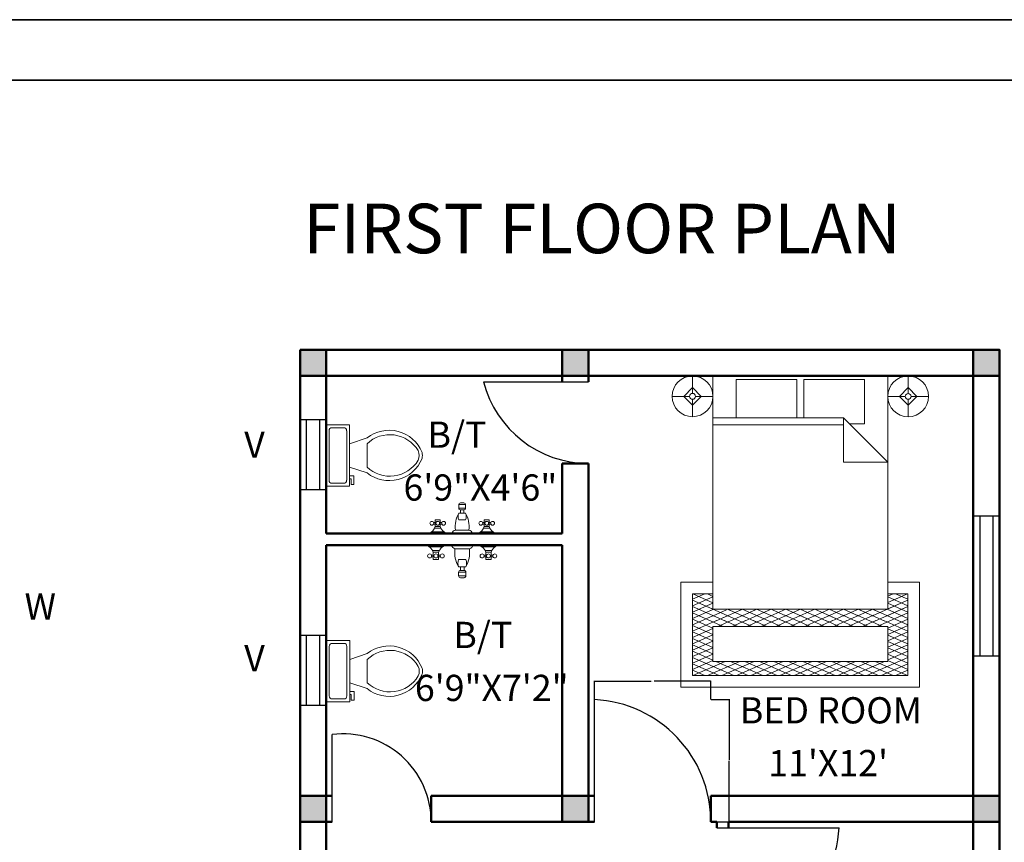
# Model space of a CAD drawing. Units: inches. Extents: x 28637 to 29820, y 17246 to 17928.
# Tile 5 of 6: x 28996 to 29334, y 17646 to 17928. Entities that reach past the tile are written whole.
import ezdxf

# ---------------------------------------------------------------- set-up
doc = ezdxf.new("R2010")
doc.units = ezdxf.units.IN
for name, color, linetype, lineweight in [('A-ANNO-DIMS', 2, 'Continuous', 18), ('A-ANNO-TEXT', 7, 'Continuous', 25), ('A-ANNO-TTLB', 7, 'Continuous', 35), ('A-AREA-IDEN', 30, 'Continuous', 25), ('A-COLS', 1, 'Continuous', 50), ('A-DOOR', 4, 'Continuous', 25), ('A-FLOR-FIXT', 8, 'Continuous', 18), ('A-FURN', 8, 'Continuous', 18), ('A-GLAZ', 4, 'Continuous', 25), ('A-WALL', 7, 'Continuous', 50)]:
    doc.layers.add(name, color=color, linetype=linetype, lineweight=lineweight)
doc.styles.get("Standard").update_dxf_attribs({"font": 'arial.ttf'})
doc.dimstyles.get("Standard").update_dxf_attribs({"dimtxt": 0.18, "dimasz": 0.18, "dimexe": 0.18, "dimexo": 0.0625, "dimgap": 0.09, "dimtad": 0, "dimtih": 1, "dimtoh": 1, "dimdec": 4, "dimzin": 0, "dimdsep": 46, "dimtxsty": 'Standard', "dimcen": 0.09, "dimadec": 0, "dimazin": 0, "dimtfac": 1, "dimtdec": 4, "dimtofl": 0, "dimtmove": 0, "dimatfit": 3, "dimfxl": 1, "dimtolj": 1, "dimtzin": 0, "dimarcsym": 0})

# ---------------------------------------------------------------- blocks, each defined once
blk = doc.blocks.new('Bed - Queen')
for p, q in [((0, -80.00003), (0, 0)), ((0, 0), (59.99999, 0)), ((59.99999, 0), (59.99999, -80.00003)), ((7.99999, -1.2), (28.79998, -1.2)), ((7.99999, -14.4), (7.99999, -1.2)), ((28.79998, -1.2), (28.79998, -14.4)), ((31.19999, -1.2), (51.99999, -1.2)), ((31.19999, -14.4), (31.19999, -1.2)), ((51.99999, -1.2), (51.99999, -16.4)), ((0, -14.4), (44.8, -14.4)), ((44.8, -16.8), (0, -16.8)), ((59.99999, -29.6), (44.8, -14.4)), ((44.8, -14.4), (44.8, -29.6)), ((51.99999, -16.4), (46.79936, -16.4)), ((44.8, -29.6), (59.99999, -29.6)), ((59.99999, -80.00003), (0, -80.00003))]:
    blk.add_line(p, q)
blk = doc.blocks.new('Lamp - Table')
for p, q in [((0, 7), (0, 1)), ((-1, 0), (-7, 0)), ((0, 3), (-3, 0)), ((-3, 0), (0, -3)), ((3, 0), (0, 3)), ((0, -3), (3, 0)), ((1, 0), (7, 0)), ((0, -1), (0, -7))]:
    blk.add_line(p, q)
for radius in [7, 1]:
    blk.add_circle((0, 0), radius)
blk = doc.blocks.new('Toilet - top')
for p, q in [((9.5, -6), (9.5, -2)), ((-10, -8.5), (-8, -8.5)), ((-10, -9.5), (-10, -8.5)), ((-7, -9.5), (-10, -9.5)), ((-8, -8.5), (-8, -8)), ((-7, -8), (-7, -9.5)), ((-4, -8), (-6, -14)), ((4, -8), (6, -14)), ((4, -14), (-4, -14))]:
    blk.add_line(p, q)
blk.add_lwpolyline([(10.5, -8), (10.5, 0), (-10.5, 0), (-10.5, -8)], close=True)
for points in [[(-9.5, -2), (-9.5, -6)], [(8.5, -1), (-8.5, -1)], [(-8.5, -7), (8.5, -7)]]:
    blk.add_lwpolyline(points)
for centre, radius, start, end in [((-8.62, -1.88), 0.884, 81.8699, 188.1301), ((8.62, -1.88), 0.884, 351.8699, 98.1301), ((-8.62, -6.12), 0.884, 171.8699, 278.1301), ((8.62, -6.12), 0.884, 261.8699, 8.1301), ((3.52, -21.58), 12.17, 141.4691, 247.9714), ((4.2, -21.82), 11.33, 136.3677, 238.9468), ((-3.52, -21.58), 12.17, 292.0284, 38.5307), ((-4.2, -21.82), 11.33, 301.053, 43.6321), ((0, -27.88), 4, 245.7318, 294.2682), ((0, -29), 4, 254.8605, 285.1395)]:
    blk.add_arc(centre, radius, start, end)
blk = doc.blocks.new('Faucet - Bathroom front')
for p, q in [((-0.5, 4.25), (0.5, 4.25)), ((0.5, 3.75), (-0.5, 3.75)), ((-0.5, 3), (0.5, 3)), ((-0.25, 3), (-0.25, 3.5)), ((0.25, 3.5), (0.25, 3)), ((-4, 1.625), (-4.25, 1.625)), ((-4, 1.375), (-4.25, 1.375)), ((-3.25, 1.625), (-3, 1.625)), ((-3.25, 1.375), (-3, 1.375)), ((0.5, 2), (-0.5, 2)), ((3.25, 1.625), (3, 1.625)), ((3.25, 1.375), (3, 1.375)), ((4, 1.625), (4.25, 1.625)), ((4, 1.375), (4.25, 1.375)), ((-5, 0), (-2.25, 0)), ((-4.5087, 0.25), (-2.7408, 0.25)), ((-3.1442, 0.75), (-4.0979, 0.75)), ((-1.5, 0), (1.5, 0)), ((-1, 0.5), (1, 0.5)), ((2.25, 0), (5, 0)), ((2.7413, 0.25), (4.5092, 0.25)), ((4.1058, 0.75), (3.1521, 0.75))]:
    blk.add_line(p, q)
for points in [[(-0.5, 3.75), (-0.5, 4.25)], [(-0.25, 4.5), (0.25, 4.5)], [(0.5, 4.25), (0.5, 3.75)], [(0.25, 3.5), (-0.25, 3.5)]]:
    blk.add_lwpolyline(points)
for points in [[(-4, 1), (-4, 2), (-3.25, 2), (-3.25, 1)], [(3.25, 1), (3.25, 2), (4, 2), (4, 1)]]:
    blk.add_lwpolyline(points, close=True)
for centre in [(-4.5, 1.5), (-3.625, 1.5), (-2.75, 1.5), (2.75, 1.5), (3.625, 1.5), (4.5, 1.5)]:
    blk.add_circle(centre, 0.2795)
for centre, radius, start, end in [((-0.2575, 4.2575), 0.2426, 88.22243, 181.7776), ((0.2575, 4.2575), 0.2426, 358.2224, 91.77757), ((3, 1), 4.0311, 150.2551, 187.125), ((0.6413, 2.5), 1.246, 156.3417, 203.6583), ((-0.2575, 3.7425), 0.2426, 178.2224, 271.7776), ((0.2575, 3.7425), 0.2426, 268.2224, 1.777565), ((-3, 1), 4.0311, 352.875, 29.74488), ((-0.6413, 2.5), 1.246, 336.3417, 23.65835), ((-5.375, 1.375), 1.4252, 285.2551, 344.7449), ((-1.875, 1.375), 1.4252, 195.2551, 254.7449), ((-0.7962, -0.2038), 0.7327, 106.1502, 163.8498), ((0.7962, -0.2038), 0.7327, 16.1502, 73.84979), ((1.875, 1.375), 1.4252, 285.2551, 344.7449), ((5.375, 1.375), 1.4252, 195.2551, 254.7449)]:
    blk.add_arc(centre, radius, start, end)
blk = doc.blocks.new('DOOR-42')
blk.add_line((28900.64, 17650.75), (28942.64, 17650.75))
blk.add_arc((28900.64, 17652.8), 42.05, 270, 357.2056)
blk = doc.blocks.new('DOOR-37')
blk.add_line((28816.64, 17803.75), (28852.64, 17803.75))
blk.add_arc((28852.64, 17812.9), 37.14, 194.25, 270)
blk = doc.blocks.new('DOOR-30')
blk.add_line((28764.64, 17652.75), (28764.64, 17682.75))
blk.add_arc((28768.41, 17652.75), 30.24, 0, 97.1527)
blk = doc.blocks.new('*D36')
at = {"layer": 'A-ANNO-DIMS', "color": 0, "lineweight": -2, "transparency": 16777216}
for p, q in [((29232.93, 17694.75), (29239.35, 17694.75)), ((29239.17, 17694.57), (29239.17, 17673.94)), ((29239.17, 17652.93), (29239.17, 17673.57)), ((29232.93, 17652.75), (29239.35, 17652.75))]:
    blk.add_line(p, q, dxfattribs=at)
at = {"layer": 'A-ANNO-DIMS', "color": 0, "transparency": 16777216}
for points in [[(29239.14, 17694.57), (29239.2, 17694.57), (29239.17, 17694.75)], [(29239.14, 17652.93), (29239.2, 17652.93), (29239.17, 17652.75)]]:
    blk.add_solid(points, dxfattribs=at)
at = {"layer": 'Defpoints', "color": 0, "transparency": 16777216}
for p in [(29232.87, 17694.75), (29239.17, 17694.75), (29232.87, 17652.75)]:
    blk.add_point(p, dxfattribs=at)
at = {"layer": 'A-ANNO-DIMS', "color": 0, "transparency": 16777216, "insert": (29239.17, 17673.75), "char_height": 0.18, "attachment_point": 5}
blk.add_mtext('\\A1;DOOR 42 TYP.', dxfattribs=at)
blk = doc.blocks.new('*D37')
at = {"layer": 'A-ANNO-DIMS', "color": 0, "lineweight": -2, "transparency": 16777216}
for p, q in [((29192.87, 17694.81), (29192.87, 17701.23)), ((29193.05, 17701.05), (29212.34, 17701.05)), ((29232.69, 17701.05), (29213.4, 17701.05)), ((29232.87, 17694.81), (29232.87, 17701.23))]:
    blk.add_line(p, q, dxfattribs=at)
at = {"layer": 'A-ANNO-DIMS', "color": 0, "transparency": 16777216}
for points in [[(29193.05, 17701.08), (29193.05, 17701.02), (29192.87, 17701.05)], [(29232.69, 17701.08), (29232.69, 17701.02), (29232.87, 17701.05)]]:
    blk.add_solid(points, dxfattribs=at)
at = {"layer": 'Defpoints', "color": 0, "transparency": 16777216}
for p in [(29192.87, 17701.05), (29192.87, 17694.75), (29232.87, 17694.75)]:
    blk.add_point(p, dxfattribs=at)
at = {"layer": 'A-ANNO-DIMS', "color": 0, "transparency": 16777216, "insert": (29212.87, 17701.05), "char_height": 0.18, "attachment_point": 5}
blk.add_mtext('\\A1;40 TYP.', dxfattribs=at)

msp = doc.modelspace()

# ---------------------------------------------------------------- hatches: boundary and pattern name
at = {"layer": 'A-COLS'}
h = msp.add_hatch(color=256, dxfattribs=at)
h.dxf.hatch_style = 1
h.paths.add_polyline_path([(29091.87, 17814.75), (29091.87, 17805.75), (29100.87, 17805.75), (29100.87, 17814.75)])
h = msp.add_hatch(color=256, dxfattribs=at)
h.dxf.hatch_style = 1
h.paths.add_polyline_path([(29181.87, 17814.75), (29181.87, 17805.75), (29190.87, 17805.75), (29190.87, 17814.75)])
h = msp.add_hatch(color=256, dxfattribs=at)
h.dxf.hatch_style = 1
h.paths.add_polyline_path([(29331.87, 17814.75), (29322.87, 17814.75), (29322.87, 17805.75), (29331.87, 17805.75)])
h = msp.add_hatch(color=256, dxfattribs=at)
h.dxf.hatch_style = 1
h.paths.add_polyline_path([(29091.87, 17661.75), (29091.87, 17652.75), (29100.87, 17652.75), (29100.87, 17661.75)])
h = msp.add_hatch(color=256, dxfattribs=at)
h.dxf.hatch_style = 1
h.paths.add_polyline_path([(29181.87, 17661.75), (29181.87, 17652.75), (29190.87, 17652.75), (29190.87, 17661.75)])
h = msp.add_hatch(color=256, dxfattribs=at)
h.dxf.hatch_style = 1
h.paths.add_polyline_path([(29322.87, 17661.75), (29322.87, 17652.75), (29331.87, 17652.75), (29331.87, 17661.75)])

# ---------------------------------------------------------------- linework, layer by layer
at = {"layer": 'A-ANNO-TTLB'}
for points in [[(28637.03, 17927.97), (29820.02, 17927.97), (29820.02, 17246.37), (28637.03, 17246.37)], [(28663.78, 17907.18), (29794.75, 17907.18), (29794.75, 17268.65), (28663.78, 17268.65)]]:
    msp.add_lwpolyline(points, close=True, dxfattribs=at)
at = {"layer": 'A-COLS'}
for points in [[(29091.87, 17814.75), (29100.87, 17814.75), (29100.87, 17805.75), (29091.87, 17805.75)], [(29181.87, 17814.75), (29190.87, 17814.75), (29190.87, 17805.75), (29181.87, 17805.75)], [(29322.87, 17814.75), (29331.87, 17814.75), (29331.87, 17805.75), (29322.87, 17805.75)], [(29091.87, 17661.75), (29100.87, 17661.75), (29100.87, 17652.75), (29091.87, 17652.75)], [(29181.87, 17661.75), (29190.87, 17661.75), (29190.87, 17652.75), (29181.87, 17652.75)], [(29322.87, 17661.75), (29331.87, 17661.75), (29331.87, 17652.75), (29322.87, 17652.75)]]:
    msp.add_lwpolyline(points, close=True, dxfattribs=at)
at = {"layer": 'A-FURN'}
for p, q in [((29222.57, 17734.98), (29233.57, 17734.98)), ((29222.57, 17734.98), (29222.57, 17698.98)), ((29293.57, 17734.98), (29304.47, 17734.98)), ((29304.47, 17734.98), (29304.47, 17698.98)), ((29226.57, 17730.98), (29233.57, 17730.98)), ((29226.57, 17730.98), (29226.57, 17702.98)), ((29226.57, 17729.14), (29230.76, 17730.98)), ((29226.57, 17726.95), (29233.57, 17730.03)), ((29226.57, 17728.85), (29233.57, 17725.77)), ((29226.7, 17730.98), (29233.57, 17727.96)), ((29228.99, 17729.97), (29233.57, 17727.96)), ((29231.67, 17730.98), (29233.57, 17730.14)), ((29231.67, 17730.98), (29233.57, 17730.14)), ((29293.57, 17730.98), (29300.47, 17730.98)), ((29293.57, 17730.19), (29295.37, 17730.98)), ((29293.57, 17728), (29300.34, 17730.98)), ((29293.57, 17728), (29300.34, 17730.98)), ((29293.57, 17728), (29300.34, 17730.98)), ((29293.57, 17729.98), (29300.47, 17726.95)), ((29293.57, 17728), (29298.05, 17729.97)), ((29293.57, 17725.82), (29300.47, 17728.85)), ((29293.57, 17725.82), (29300.47, 17728.85)), ((29296.28, 17730.98), (29300.47, 17729.14)), ((29300.47, 17730.98), (29300.47, 17702.98)), ((29226.57, 17724.77), (29233.57, 17727.84)), ((29226.57, 17726.66), (29233.57, 17723.59)), ((29226.57, 17722.58), (29233.57, 17725.66)), ((29227.38, 17726.31), (29237.92, 17721.68)), ((29228.18, 17728.14), (29238.73, 17723.51)), ((29232.84, 17725.34), (29233.78, 17725.75)), ((29233.65, 17723.51), (29238.19, 17725.51)), ((29233.65, 17723.51), (29238.19, 17725.51)), ((29234.45, 17721.68), (29243.72, 17725.75)), ((29238.59, 17725.75), (29248.61, 17721.35)), ((29238.59, 17725.75), (29239.53, 17725.34)), ((29242.78, 17725.34), (29243.72, 17725.75)), ((29243.58, 17723.51), (29248.61, 17725.72)), ((29243.58, 17723.51), (29248.13, 17725.51)), ((29243.64, 17725.72), (29251.1, 17722.44)), ((29244.39, 17721.68), (29253.58, 17725.72)), ((29248.53, 17725.75), (29253.64, 17723.51)), ((29249.36, 17721.68), (29258.63, 17725.75)), ((29253.5, 17725.75), (29254.44, 17725.34)), ((29254.06, 17725.51), (29258.61, 17723.51)), ((29254.33, 17721.68), (29263.6, 17725.75)), ((29258.55, 17725.72), (29266.01, 17722.44)), ((29259.3, 17721.68), (29268.57, 17725.75)), ((29263.52, 17725.72), (29268.55, 17723.51)), ((29264.27, 17721.68), (29273.54, 17725.75)), ((29268.49, 17725.72), (29275.95, 17722.44)), ((29269.24, 17721.68), (29278.43, 17725.72)), ((29273.46, 17725.72), (29278.49, 17723.51)), ((29278.35, 17725.75), (29283.46, 17723.51)), ((29278.37, 17723.51), (29282.92, 17725.51)), ((29282.54, 17725.34), (29283.48, 17725.75)), ((29283.34, 17723.51), (29287.89, 17725.51)), ((29283.4, 17725.72), (29288.43, 17723.51)), ((29283.88, 17725.51), (29288.43, 17723.51)), ((29287.51, 17725.34), (29288.45, 17725.75)), ((29288.29, 17725.75), (29289.23, 17725.34)), ((29288.31, 17723.51), (29298.86, 17728.14)), ((29288.31, 17723.51), (29298.86, 17728.14)), ((29288.37, 17725.72), (29300.47, 17720.4)), ((29289.12, 17721.68), (29299.66, 17726.31)), ((29293.34, 17725.72), (29300.47, 17722.58)), ((29293.57, 17727.8), (29300.47, 17724.77)), ((29293.57, 17723.63), (29300.47, 17726.66)), ((29294.38, 17725.26), (29300.47, 17722.58)), ((29294.38, 17725.26), (29300.47, 17722.58)), ((29226.57, 17724.48), (29237.12, 17719.84)), ((29226.57, 17720.4), (29233.57, 17723.48)), ((29226.57, 17722.3), (29233.57, 17719.22)), ((29226.57, 17718.21), (29234.83, 17721.84)), ((29234.45, 17721.68), (29239, 17723.68)), ((29234.45, 17721.68), (29239, 17723.68)), ((29235.25, 17719.84), (29239.8, 17721.84)), ((29237.54, 17721.84), (29242.09, 17719.84)), ((29238.67, 17723.53), (29247.06, 17719.84)), ((29239.42, 17721.68), (29243.97, 17723.68)), ((29240.22, 17719.84), (29244.77, 17721.84)), ((29245.19, 17719.84), (29249.74, 17721.84)), ((29247.48, 17721.84), (29252.03, 17719.84)), ((29248.28, 17723.68), (29252.83, 17721.68)), ((29250.16, 17719.84), (29254.71, 17721.84)), ((29250.16, 17719.84), (29254.71, 17721.84)), ((29250.16, 17719.84), (29254.71, 17721.84)), ((29252.45, 17721.84), (29257, 17719.84)), ((29252.45, 17721.84), (29257, 17719.84)), ((29253.25, 17723.68), (29257.8, 17721.68)), ((29255.13, 17719.84), (29259.68, 17721.84)), ((29257.42, 17721.84), (29261.97, 17719.84)), ((29258.22, 17723.68), (29262.77, 17721.68)), ((29260.1, 17719.84), (29264.65, 17721.84)), ((29262.39, 17721.84), (29266.94, 17719.84)), ((29263.19, 17723.68), (29267.74, 17721.68)), ((29265.07, 17719.84), (29269.62, 17721.84)), ((29267.36, 17721.84), (29271.91, 17719.84)), ((29268.16, 17723.68), (29272.71, 17721.68)), ((29270.04, 17719.84), (29274.59, 17721.84)), ((29272.33, 17721.84), (29276.88, 17719.84)), ((29273.13, 17723.68), (29277.68, 17721.68)), ((29274.21, 17721.68), (29278.76, 17723.68)), ((29275.01, 17719.84), (29279.56, 17721.84)), ((29275.01, 17719.84), (29279.56, 17721.84)), ((29275.01, 17719.84), (29279.56, 17721.84)), ((29277.3, 17721.84), (29281.85, 17719.84)), ((29278.1, 17723.68), (29282.65, 17721.68)), ((29279.18, 17721.68), (29283.73, 17723.68)), ((29279.98, 17719.84), (29284.53, 17721.84)), ((29279.98, 17719.84), (29284.53, 17721.84)), ((29282.27, 17721.84), (29286.82, 17719.84)), ((29283.07, 17723.68), (29287.62, 17721.68)), ((29284.15, 17721.68), (29288.7, 17723.68)), ((29284.15, 17721.68), (29288.7, 17723.68)), ((29284.95, 17719.84), (29289.5, 17721.84)), ((29287.24, 17721.84), (29291.79, 17719.84)), ((29288.04, 17723.68), (29292.59, 17721.68)), ((29288.04, 17723.68), (29292.59, 17721.68)), ((29289.92, 17719.84), (29300.47, 17724.48)), ((29292.21, 17721.84), (29300.47, 17718.21)), ((29293.01, 17723.68), (29300.47, 17720.4)), ((29293.57, 17719.26), (29300.47, 17722.3)), ((29226.57, 17720.11), (29233.57, 17717.03)), ((29226.57, 17716.03), (29233.57, 17719.11)), ((29233.57, 17719.84), (29293.57, 17719.84)), ((29233.57, 17719.84), (29233.57, 17707.84)), ((29293.57, 17717.08), (29300.47, 17720.11)), ((29293.57, 17719.84), (29293.57, 17707.84)), ((29293.57, 17719.06), (29300.47, 17716.03)), ((29226.57, 17717.93), (29233.57, 17714.85)), ((29226.57, 17713.84), (29233.57, 17716.92)), ((29226.57, 17715.74), (29233.57, 17712.66)), ((29293.57, 17714.9), (29300.47, 17717.93)), ((29293.57, 17716.87), (29300.47, 17713.84)), ((29293.57, 17712.71), (29300.47, 17715.74)), ((29226.57, 17711.66), (29233.57, 17714.74)), ((29226.57, 17713.56), (29233.57, 17710.48)), ((29226.57, 17709.47), (29233.57, 17712.55)), ((29293.57, 17714.69), (29300.47, 17711.66)), ((29293.57, 17710.53), (29300.47, 17713.56)), ((29293.57, 17712.51), (29300.47, 17709.47)), ((29226.57, 17711.37), (29233.57, 17708.29)), ((29226.57, 17707.29), (29233.57, 17710.37)), ((29226.57, 17709.19), (29240.7, 17702.98)), ((29226.57, 17705.11), (29233.57, 17708.18)), ((29286.34, 17702.98), (29300.47, 17709.19)), ((29293.57, 17708.34), (29300.47, 17711.37)), ((29293.57, 17710.32), (29300.47, 17707.29)), ((29293.57, 17708.14), (29300.47, 17705.11)), ((29226.57, 17707), (29235.73, 17702.98)), ((29226.57, 17704.82), (29230.76, 17702.98)), ((29226.7, 17702.98), (29237.78, 17707.84)), ((29231.67, 17702.98), (29242.75, 17707.84)), ((29233.57, 17707.84), (29293.57, 17707.84)), ((29234.6, 17707.84), (29245.67, 17702.98)), ((29236.64, 17702.98), (29247.72, 17707.84)), ((29236.64, 17702.98), (29247.72, 17707.84)), ((29236.64, 17702.98), (29247.72, 17707.84)), ((29239.57, 17707.84), (29250.64, 17702.98)), ((29241.61, 17702.98), (29252.69, 17707.84)), ((29241.61, 17702.98), (29252.69, 17707.84)), ((29244.54, 17707.84), (29255.61, 17702.98)), ((29246.58, 17702.98), (29257.66, 17707.84)), ((29249.51, 17707.84), (29260.58, 17702.98)), ((29251.55, 17702.98), (29262.63, 17707.84)), ((29254.48, 17707.84), (29265.55, 17702.98)), ((29256.52, 17702.98), (29267.6, 17707.84)), ((29259.45, 17707.84), (29270.52, 17702.98)), ((29261.49, 17702.98), (29272.57, 17707.84)), ((29264.42, 17707.84), (29275.49, 17702.98)), ((29266.46, 17702.98), (29277.53, 17707.84)), ((29269.39, 17707.84), (29280.46, 17702.98)), ((29271.43, 17702.98), (29282.5, 17707.84)), ((29274.36, 17707.84), (29285.43, 17702.98)), ((29276.4, 17702.98), (29287.47, 17707.84)), ((29279.33, 17707.84), (29290.4, 17702.98)), ((29281.37, 17702.98), (29292.44, 17707.84)), ((29284.3, 17707.84), (29295.37, 17702.98)), ((29284.3, 17707.84), (29295.37, 17702.98)), ((29289.27, 17707.84), (29300.34, 17702.98)), ((29291.31, 17702.98), (29300.47, 17707)), ((29296.28, 17702.98), (29300.47, 17704.82)), ((29226.57, 17702.98), (29300.47, 17702.98)), ((29222.57, 17698.98), (29304.47, 17698.98))]:
    msp.add_line(p, q, dxfattribs=at)
at = {"layer": 'A-GLAZ'}
for p, q in [((29100.87, 17790.75), (29091.87, 17790.75)), ((29094.12, 17766.75), (29094.12, 17790.75)), ((29098.62, 17766.75), (29098.62, 17790.75)), ((29100.87, 17766.75), (29091.87, 17766.75)), ((29322.87, 17757.75), (29331.87, 17757.75)), ((29325.12, 17757.75), (29325.12, 17709.75)), ((29329.62, 17757.75), (29329.62, 17709.75)), ((29100.87, 17716.75), (29091.87, 17716.75)), ((29094.12, 17692.75), (29094.12, 17716.75)), ((29098.62, 17692.75), (29098.62, 17716.75)), ((29322.87, 17709.75), (29331.87, 17709.75)), ((29100.87, 17692.75), (29091.87, 17692.75))]:
    msp.add_line(p, q, dxfattribs=at)
at = {"layer": 'A-WALL'}
for p, q in [((29091.87, 17814.75), (29331.87, 17814.75)), ((29091.87, 17334.75), (29091.87, 17814.75)), ((29190.87, 17814.75), (29190.87, 17803.75)), ((29331.87, 17814.75), (29331.87, 17334.75)), ((29100.87, 17805.75), (29181.87, 17805.75)), ((29100.87, 17751.75), (29100.87, 17805.75)), ((29181.87, 17805.75), (29181.87, 17803.75)), ((29181.87, 17805.75), (29181.87, 17803.75)), ((29190.87, 17805.75), (29322.87, 17805.75)), ((29190.87, 17805.75), (29190.87, 17803.75)), ((29322.87, 17805.75), (29322.87, 17661.75)), ((29322.87, 17805.75), (29322.87, 17661.75)), ((29181.87, 17775.75), (29190.87, 17775.75)), ((29181.87, 17775.75), (29181.87, 17751.75)), ((29181.87, 17775.75), (29181.87, 17751.75)), ((29190.87, 17775.75), (29190.87, 17661.75)), ((29190.87, 17775.75), (29190.87, 17661.75)), ((29100.87, 17751.75), (29181.87, 17751.75)), ((29100.87, 17747.75), (29181.87, 17747.75)), ((29100.87, 17661.75), (29100.87, 17747.75)), ((29181.87, 17747.75), (29181.87, 17661.75)), ((29181.87, 17747.75), (29181.87, 17661.75)), ((29100.87, 17661.75), (29102.87, 17661.75)), ((29136.87, 17661.75), (29181.87, 17661.75)), ((29136.87, 17652.75), (29136.87, 17661.75)), ((29190.87, 17661.75), (29192.87, 17661.75)), ((29232.87, 17661.75), (29322.87, 17661.75)), ((29232.87, 17661.75), (29232.87, 17652.75)), ((29100.87, 17652.75), (29102.87, 17652.75)), ((29100.87, 17508.75), (29100.87, 17652.75)), ((29136.87, 17652.75), (29192.87, 17652.75)), ((29232.87, 17652.75), (29234.87, 17652.75)), ((29232.87, 17652.75), (29234.87, 17652.75)), ((29234.87, 17652.75), (29234.87, 17650.75)), ((29238.87, 17652.75), (29238.87, 17650.75)), ((29238.87, 17652.75), (29322.87, 17652.75)), ((29322.87, 17652.75), (29322.87, 17484.75)), ((29322.87, 17652.75), (29322.87, 17484.75))]:
    msp.add_line(p, q, dxfattribs=at)

# ---------------------------------------------------------------- block references
at = {"layer": 'A-DOOR'}
for name, p in [('DOOR-37', (338.22, 0)), ('DOOR-30', (338.22, 0)), ('DOOR-42', (334.22, 0))]:
    msp.add_blockref(name, p, dxfattribs=at)
at = {"layer": 'A-DOOR', "rotation": 90.00000000000261}
msp.add_blockref('DOOR-42', (46843.62, -11247.89), dxfattribs=at)
at = {"layer": 'A-FLOR-FIXT', "rotation": 90}
for p in [(29100.86, 17778.49), (29100.89, 17704.5)]:
    msp.add_blockref('Toilet - top', p, dxfattribs=at)
at = {"layer": 'A-FLOR-FIXT', "xscale": 2.319878252974637, "yscale": 2.319878252974637, "zscale": 2.319878252974637}
msp.add_blockref('Faucet - Bathroom front', (29147.51, 17751.75), dxfattribs=at)
at = {"layer": 'A-FLOR-FIXT', "xscale": -2.485809345179645, "yscale": 2.485809345179645, "zscale": 2.485809345179645, "rotation": 180}
msp.add_blockref('Faucet - Bathroom front', (29147.51, 17747.75), dxfattribs=at)
at = {"layer": 'A-FURN'}
for name, p in [('Lamp - Table', (29226.57, 17798.77)), ('Bed - Queen', (29233.57, 17805.75)), ('Lamp - Table', (29300.57, 17798.75))]:
    msp.add_blockref(name, p, dxfattribs=at)

# ---------------------------------------------------------------- texts
at = {"layer": 'A-ANNO-TEXT'}
for s, height, p in [('   FIRST FLOOR PLAN', 17, (29077.33, 17847.85)), ('    V', 9, (29061.69, 17777.69)), ('    W', 9, (28986.3, 17722.18)), ('    V', 9, (29061.69, 17704.44))]:
    msp.add_text(s, height=height, dxfattribs=at).set_placement(p)
at = {"layer": 'A-AREA-IDEN'}
for s, p in [('    B/T', (29124.61, 17781.11)), (' 6\'9"X4\'6"', (29124.61, 17762.99)), ('   B/T', (29136.21, 17712.42)), ('6\'9"X7\'2"', (29131.27, 17694.24)), ('BED ROOM', (29242.8, 17686.56)), (" 11'X12'", (29249.79, 17668.45))]:
    msp.add_text(s, height=9, dxfattribs=at).set_placement(p)

# ---------------------------------------------------------------- dimensions: what is measured, and where the dimension line sits
at = {"layer": 'A-ANNO-DIMS'}
for base, p1, p2, angle, text, picture, middle in [((29192.87, 17701.05), (29232.87, 17694.75), (29192.87, 17694.75), 180, '<> TYP.', '*D37', (29212.87, 17701.05)), ((29239.17, 17694.75), (29232.87, 17652.75), (29232.87, 17694.75), 90, 'DOOR <> TYP.', '*D36', (29239.17, 17673.75))]:
    dim = msp.add_linear_dim(base=base, p1=p1, p2=p2, angle=angle, text=text, dimstyle='Standard', override={"dimdec": 0, "dimlfac": 1, "dimrnd": 0, "dimzin": 0, "dimdsep": 46, "dimlunit": 2}, dxfattribs=at)
    dim.commit()
    dim.dimension.update_dxf_attribs({"geometry": picture, "text_midpoint": middle})

doc.saveas('drawing.dxf')
